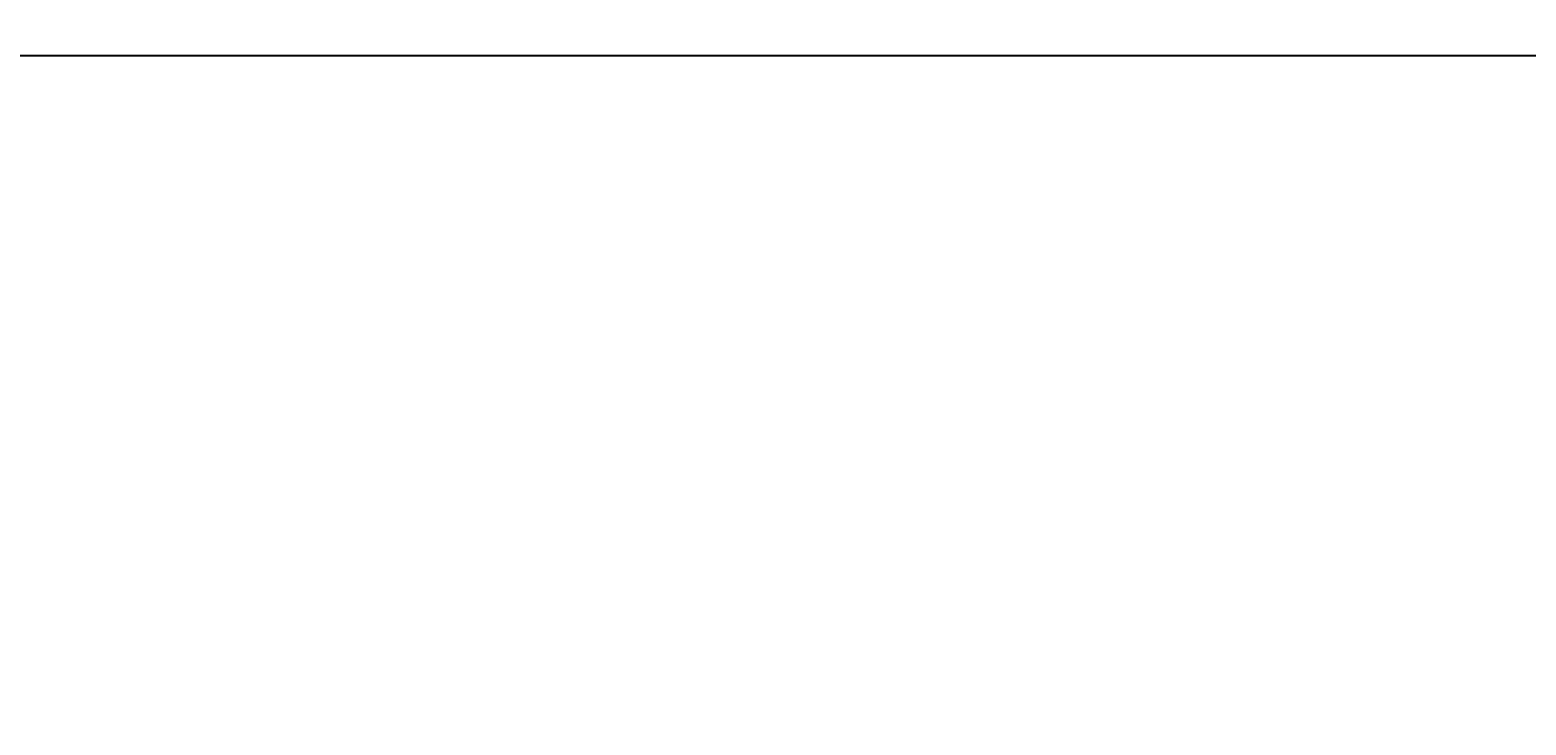
# Model space of a CAD drawing. Units: inches. Extents: x 35362 to 73946, y 43607 to 67532.
# Tile 116 of 134: x 50761 to 50905, y 49195 to 49262. Entities that reach past the tile are written whole.
import ezdxf

# ---------------------------------------------------------------- set-up
doc = ezdxf.new("R2010")
doc.units = ezdxf.units.IN
doc.header["$MEASUREMENT"] = 0
doc.layers.add('A-ANNO-DIMS', color=2, linetype='Continuous', lineweight=18)
doc.styles.get("Standard").update_dxf_attribs({"font": 'arial.ttf'})
doc.dimstyles.get("Standard").update_dxf_attribs({"dimtxt": 0.18, "dimasz": 0.18, "dimexe": 0.18, "dimexo": 0.0625, "dimgap": 0.09, "dimtad": 0, "dimtih": 1, "dimtoh": 1, "dimdec": 4, "dimzin": 0, "dimdsep": 46, "dimtxsty": 'Standard', "dimcen": 0.09, "dimadec": 0, "dimazin": 0, "dimtfac": 1, "dimtdec": 4, "dimtofl": 0, "dimtmove": 0, "dimatfit": 3, "dimfxl": 1, "dimtolj": 1, "dimtzin": 0, "dimarcsym": 0})

# ---------------------------------------------------------------- blocks, each defined once
blk = doc.blocks.new('*D11')
at = {"layer": 'A-ANNO-DIMS', "color": 0, "lineweight": -2, "transparency": 16777216}
for p, q in [((47978.66, 56028.77), (47978.66, 43606.68)), ((53109.76, 56028.77), (53109.76, 43606.68)), ((47978.84, 43606.86), (50543.87, 43606.86)), ((53109.58, 43606.86), (50544.55, 43606.86))]:
    blk.add_line(p, q, dxfattribs=at)
at = {"layer": 'A-ANNO-DIMS', "color": 0, "transparency": 16777216}
for points in [[(47978.84, 43606.89), (47978.84, 43606.83), (47978.66, 43606.86)], [(53109.58, 43606.89), (53109.58, 43606.83), (53109.76, 43606.86)]]:
    blk.add_solid(points, dxfattribs=at)
at = {"layer": 'Defpoints', "color": 0, "transparency": 16777216}
for p in [(47978.66, 56028.84), (53109.76, 56028.84), (53109.76, 43606.86)]:
    blk.add_point(p, dxfattribs=at)
at = {"layer": 'A-ANNO-DIMS', "color": 0, "transparency": 16777216, "insert": (50544.21, 43606.86), "char_height": 0.18, "attachment_point": 5}
blk.add_mtext('\\A1;5131', dxfattribs=at)
blk = doc.blocks.new('*D13')
at = {"layer": 'A-ANNO-DIMS', "color": 0, "lineweight": -2, "transparency": 16777216}
for p, q in [((48373.49, 51694.02), (48373.49, 43606.68)), ((51029.04, 51694.02), (51029.04, 43606.68)), ((48373.67, 43606.86), (49700.8, 43606.86)), ((51028.86, 43606.86), (49701.73, 43606.86))]:
    blk.add_line(p, q, dxfattribs=at)
at = {"layer": 'A-ANNO-DIMS', "color": 0, "transparency": 16777216}
for points in [[(48373.67, 43606.89), (48373.67, 43606.83), (48373.49, 43606.86)], [(51028.86, 43606.89), (51028.86, 43606.83), (51029.04, 43606.86)]]:
    blk.add_solid(points, dxfattribs=at)
at = {"layer": 'Defpoints', "color": 0, "transparency": 16777216}
for p in [(48373.49, 51694.09), (51029.04, 51694.09), (51029.04, 43606.86)]:
    blk.add_point(p, dxfattribs=at)
at = {"layer": 'A-ANNO-DIMS', "color": 0, "transparency": 16777216, "insert": (49701.27, 43606.86), "char_height": 0.18, "attachment_point": 5}
blk.add_mtext('\\A1;2655.6', dxfattribs=at)
blk = doc.blocks.new('*D17')
at = {"layer": 'A-ANNO-DIMS', "color": 0, "lineweight": -2, "transparency": 16777216}
for p, q in [((49923.31, 61293.22), (49923.31, 43606.68)), ((51913.93, 61293.22), (51913.93, 43606.68)), ((49923.49, 43606.86), (50918.16, 43606.86)), ((51913.75, 43606.86), (50919.07, 43606.86))]:
    blk.add_line(p, q, dxfattribs=at)
at = {"layer": 'A-ANNO-DIMS', "color": 0, "transparency": 16777216}
for points in [[(49923.49, 43606.89), (49923.49, 43606.83), (49923.31, 43606.86)], [(51913.75, 43606.89), (51913.75, 43606.83), (51913.93, 43606.86)]]:
    blk.add_solid(points, dxfattribs=at)
at = {"layer": 'Defpoints', "color": 0, "transparency": 16777216}
for p in [(49923.31, 61293.29), (51913.93, 61293.29), (51913.93, 43606.86)]:
    blk.add_point(p, dxfattribs=at)
at = {"layer": 'A-ANNO-DIMS', "color": 0, "transparency": 16777216, "insert": (50918.62, 43606.86), "char_height": 0.18, "attachment_point": 5}
blk.add_mtext('\\A1;1990.6', dxfattribs=at)
blk = doc.blocks.new('*D67')
at = {"layer": 'A-ANNO-DIMS', "color": 0, "lineweight": -2, "transparency": 16777216}
for p, q in [((56873.54, 53351.53), (35361.77, 53351.53)), ((35361.95, 53351.35), (35361.95, 49400.89)), ((35361.95, 45450.07), (35361.95, 49400.53)), ((53793.58, 45449.89), (35361.77, 45449.89))]:
    blk.add_line(p, q, dxfattribs=at)
at = {"layer": 'A-ANNO-DIMS', "color": 0, "transparency": 16777216}
for points in [[(35361.92, 53351.35), (35361.98, 53351.35), (35361.95, 53351.53)], [(35361.92, 45450.07), (35361.98, 45450.07), (35361.95, 45449.89)]]:
    blk.add_solid(points, dxfattribs=at)
at = {"layer": 'Defpoints', "color": 0, "transparency": 16777216}
for p in [(35361.95, 53351.53), (56873.6, 53351.53), (53793.64, 45449.89)]:
    blk.add_point(p, dxfattribs=at)
at = {"layer": 'A-ANNO-DIMS', "color": 0, "transparency": 16777216, "insert": (35361.95, 49400.71), "char_height": 0.18, "attachment_point": 5}
blk.add_mtext('\\A1;7901.6', dxfattribs=at)
blk = doc.blocks.new('*D84')
at = {"layer": 'A-ANNO-DIMS', "color": 0, "lineweight": -2, "transparency": 16777216}
for p, q in [((55540.23, 49259.94), (35361.77, 49259.94)), ((35361.95, 49259.76), (35361.95, 49115.14)), ((35361.95, 48970.16), (35361.95, 49114.78)), ((55540.23, 48969.98), (35361.77, 48969.98))]:
    blk.add_line(p, q, dxfattribs=at)
at = {"layer": 'A-ANNO-DIMS', "color": 0, "transparency": 16777216}
for points in [[(35361.92, 49259.76), (35361.98, 49259.76), (35361.95, 49259.94)], [(35361.92, 48970.16), (35361.98, 48970.16), (35361.95, 48969.98)]]:
    blk.add_solid(points, dxfattribs=at)
at = {"layer": 'Defpoints', "color": 0, "transparency": 16777216}
for p in [(35361.95, 49259.94), (55540.3, 49259.94), (55540.3, 48969.98)]:
    blk.add_point(p, dxfattribs=at)
at = {"layer": 'A-ANNO-DIMS', "color": 0, "transparency": 16777216, "insert": (35361.95, 49114.96), "char_height": 0.18, "attachment_point": 5}
blk.add_mtext('\\A1;289.96', dxfattribs=at)
blk = doc.blocks.new('*D86')
at = {"layer": 'A-ANNO-DIMS', "color": 0, "lineweight": -2, "transparency": 16777216}
for p, q in [((51285.53, 49320.08), (35361.77, 49320.08)), ((35361.95, 49319.9), (35361.95, 49120.26)), ((35361.95, 48920.26), (35361.95, 49119.9)), ((51285.53, 48920.08), (35361.77, 48920.08))]:
    blk.add_line(p, q, dxfattribs=at)
at = {"layer": 'A-ANNO-DIMS', "color": 0, "transparency": 16777216}
for points in [[(35361.92, 49319.9), (35361.98, 49319.9), (35361.95, 49320.08)], [(35361.92, 48920.26), (35361.98, 48920.26), (35361.95, 48920.08)]]:
    blk.add_solid(points, dxfattribs=at)
at = {"layer": 'Defpoints', "color": 0, "transparency": 16777216}
for p in [(35361.95, 49320.08), (51285.59, 49320.08), (51285.59, 48920.08)]:
    blk.add_point(p, dxfattribs=at)
at = {"layer": 'A-ANNO-DIMS', "color": 0, "transparency": 16777216, "insert": (35361.95, 49120.08), "char_height": 0.18, "attachment_point": 5}
blk.add_mtext('\\A1;400.0', dxfattribs=at)
blk = doc.blocks.new('*D107')
at = {"layer": 'A-ANNO-DIMS', "color": 0, "lineweight": -2, "transparency": 16777216}
for p, q in [((50139.56, 59850.01), (50139.56, 43606.68)), ((51320.81, 59850.01), (51320.81, 43606.68)), ((50139.74, 43606.86), (50729.73, 43606.86)), ((51320.63, 43606.86), (50730.64, 43606.86))]:
    blk.add_line(p, q, dxfattribs=at)
at = {"layer": 'A-ANNO-DIMS', "color": 0, "transparency": 16777216}
for points in [[(50139.74, 43606.89), (50139.74, 43606.83), (50139.56, 43606.86)], [(51320.63, 43606.89), (51320.63, 43606.83), (51320.81, 43606.86)]]:
    blk.add_solid(points, dxfattribs=at)
at = {"layer": 'Defpoints', "color": 0, "transparency": 16777216}
for p in [(50139.56, 59850.08), (51320.81, 59850.08), (51320.81, 43606.86)]:
    blk.add_point(p, dxfattribs=at)
at = {"layer": 'A-ANNO-DIMS', "color": 0, "transparency": 16777216, "insert": (50730.19, 43606.86), "char_height": 0.18, "attachment_point": 5}
blk.add_mtext('\\A1;1181.3', dxfattribs=at)

msp = doc.modelspace()

# ---------------------------------------------------------------- dimensions: what is measured, and where the dimension line sits
at = {"layer": 'A-ANNO-DIMS'}
for base, p1, p2, override, picture, middle in [((51913.931, 43606.859), (49923.307, 61293.286), (51913.931, 61293.286), {"dimdec": 1, "dimlfac": 1, "dimrnd": 0, "dimzin": 0, "dimdsep": 46, "dimlunit": 2}, '*D17', (50918.619, 43606.859)), ((51320.8133, 43606.859), (50139.5627, 59850.0769), (51320.8133, 59850.0769), {"dimdec": 1, "dimlfac": 1, "dimrnd": 0, "dimzin": 0, "dimdsep": 46, "dimlunit": 2}, '*D107', (50730.188, 43606.859)), ((53109.76, 43606.859), (47978.665, 56028.836), (53109.76, 56028.836), {"dimdec": 0, "dimlfac": 1, "dimrnd": 0, "dimzin": 0, "dimdsep": 46, "dimlunit": 2}, '*D11', (50544.212, 43606.859)), ((51029.043, 43606.859), (48373.492, 51694.087), (51029.043, 51694.087), {"dimdec": 1, "dimlfac": 1, "dimrnd": 0, "dimzin": 0, "dimdsep": 46, "dimlunit": 2}, '*D13', (49701.267, 43606.859))]:
    dim = msp.add_linear_dim(base=base, p1=p1, p2=p2, dimstyle='Standard', override=override, dxfattribs=at)
    dim.commit()
    dim.dimension.update_dxf_attribs({"geometry": picture, "text_midpoint": middle})
for base, p1, p2, override, picture, middle in [((35361.949, 53351.529), (53793.638, 45449.894), (56873.602, 53351.529), {"dimdec": 1, "dimlfac": 1, "dimrnd": 0, "dimzin": 0, "dimdsep": 46, "dimlunit": 2}, '*D67', (35361.949, 49400.712)), ((35361.949, 49320.079), (51285.595, 48920.079), (51285.595, 49320.079), {"dimdec": 1, "dimlfac": 1, "dimrnd": 0, "dimzin": 0, "dimdsep": 46, "dimlunit": 2}, '*D86', (35361.949, 49120.079)), ((35361.9491, 49259.9353), (55540.2972, 48969.9796), (55540.2972, 49259.9353), {"dimdec": 2, "dimlfac": 1, "dimrnd": 0, "dimzin": 0, "dimdsep": 46, "dimlunit": 2}, '*D84', (35361.9491, 49114.9575))]:
    dim = msp.add_linear_dim(base=base, p1=p1, p2=p2, angle=90, dimstyle='Standard', override=override, dxfattribs=at)
    dim.commit()
    dim.dimension.update_dxf_attribs({"geometry": picture, "text_midpoint": middle})

doc.saveas('drawing.dxf')
